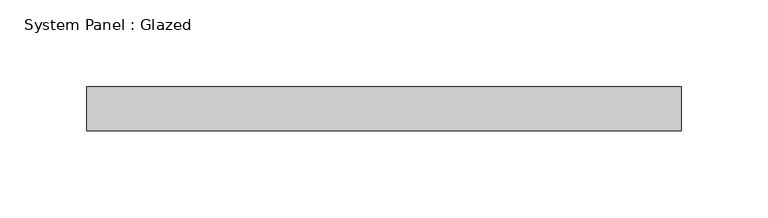
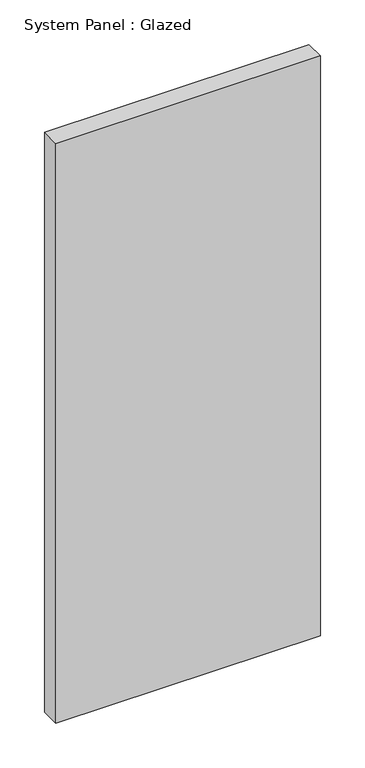
"""IFC4 building model written with IfcOpenShell, lengths in millimetres: plate geometry, System Panel : Glazed."""

from ifc_helpers import new_model, si_unit, origin, origin_with_axes, place, context, project, spatial, polyline, outline, extrude, source, transform, mapped, element, save


def system_panel_glazed_603fb926(model_context):
    return source(origin(), model_context, "Body", "SweptSolid", [
        extrude(outline(polyline([(171.45, 19.05), (-171.45, 19.05), (-171.45, 44.45), (171.45, 44.45), (171.45, 19.05)])), origin_with_axes(), (0.0, 0.0, 1.0), 793.75),
    ])


if __name__ == "__main__":
    model = new_model("IFC4")
    model_context = context("Model", 3, world=origin())
    ifc_project = project(units=[si_unit("LENGTHUNIT", "METRE", prefix="MILLI")], contexts=[model_context])
    site = spatial("IfcSite", under=ifc_project)
    building = spatial("IfcBuilding", under=site)
    placement = place(None, origin())
    system_panel_glazed_shape = system_panel_glazed_603fb926(model_context)
    element("IfcPlate", 1, ObjectType="System Panel : Glazed", at=placement, inside=building, context=model_context, shape_type="MappedRepresentation", body=[
        mapped(system_panel_glazed_shape, transform((0.0, 0.0, 0.0), x_axis=(1.0, 0.0, 0.0), y_axis=(0.0, 1.0, 0.0), z_axis=(0.0, 0.0, 1.0))),
    ])
    save(model, "model.ifc")

# Revit data of these elements
# Type "System Panel : Glazed"
#   Construction Type Id = "GSP4R"
#   Analytic Construction = "1/8 in Pilkington single glazing"
#   Visual Light Transmittance = 0.9
#   Solar Heat Gain Coefficient = 0.86
#   Heat Transfer Coefficient (U) = 1.18115 BTU/(h·ft²·°F)
# Element 1 (IfcPlate, "System Panel : Glazed")
#   Materials on its faces: "Glass"
# Materials
#   "Glass": class "Glass", colour RGB 0 128 192, transparency 0.75, Description = "Soda Lime Glass", Cost = 0
